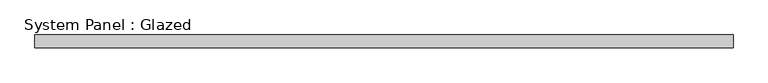
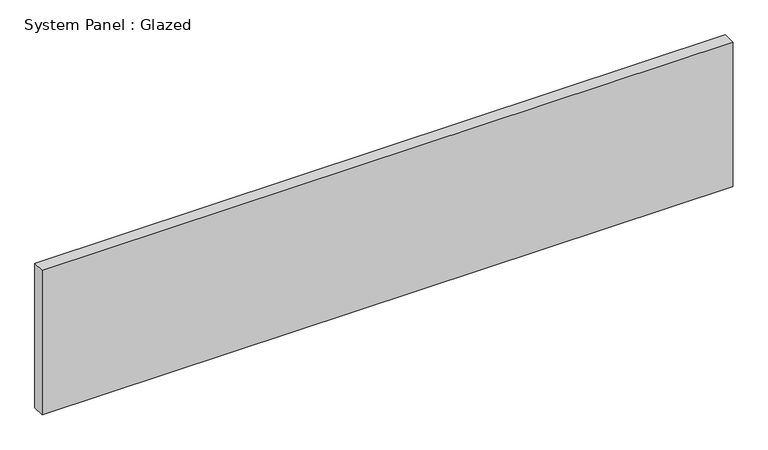
"""IFC4 building model written with IfcOpenShell, lengths in millimetres: plate geometry, System Panel : Glazed."""

from ifc_helpers import new_model, si_unit, origin, origin_with_axes, place, context, project, spatial, polyline, outline, extrude, source, transform, mapped, element, save


def system_panel_glazed_57209e1b(model_context):
    return source(origin(), model_context, "Body", "SweptSolid", [
        extrude(outline(polyline([(689.5750002, 24.5), (-689.5750002, 24.5), (-689.5750002, 49.5), (689.5750002, 49.5), (689.5750002, 24.5)])), origin_with_axes(), (0.0, 0.0, 1.0), 304.8),
    ])


if __name__ == "__main__":
    model = new_model("IFC4")
    model_context = context("Model", 3, world=origin())
    ifc_project = project(units=[si_unit("LENGTHUNIT", "METRE", prefix="MILLI")], contexts=[model_context])
    site = spatial("IfcSite", under=ifc_project)
    building = spatial("IfcBuilding", under=site)
    placement = place(None, origin())
    system_panel_glazed_shape = system_panel_glazed_57209e1b(model_context)
    element("IfcPlate", 1, ObjectType="System Panel : Glazed", at=placement, inside=building, context=model_context, shape_type="MappedRepresentation", body=[
        mapped(system_panel_glazed_shape, transform((0.0, 0.0, 0.0), x_axis=(1.0, 0.0, 0.0), y_axis=(0.0, 1.0, 0.0), z_axis=(0.0, 0.0, 1.0))),
    ])
    save(model, "model.ifc")

# Revit data of these elements
# Type "System Panel : Glazed"
#   Keynote = "H11"
#   Construction Type Id = "GSP4R"
#   Analytic Construction = "1/8 in Pilkington single glazing"
#   Visual Light Transmittance = 0.9
#   Solar Heat Gain Coefficient = 0.86
#   Heat Transfer Coefficient (U) = 6.7069 W/(m²·K)
#   Define Thermal Properties by = 1
# Element 1 (IfcPlate, "System Panel : Glazed")
#   Materials on its faces: "Glass"
# Materials
#   "Glass": class "Glass", colour RGB 0 128 192, transparency 0.9, Description = "Soda Lime Glass", Cost = 0
